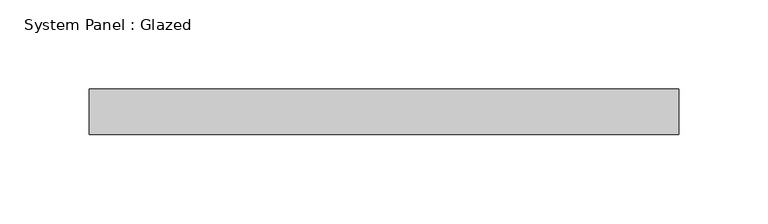
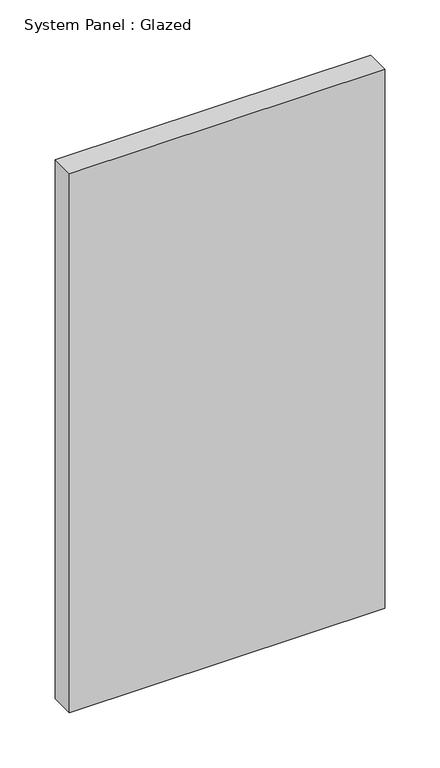
"""IFC4 building model written with IfcOpenShell, lengths in millimetres: plate geometry, System Panel : Glazed."""

from ifc_helpers import new_model, si_unit, origin, origin_with_axes, place, context, project, spatial, polyline, outline, extrude, source, transform, mapped, element, save


def system_panel_glazed_8f64e07d(model_context):
    return source(origin(), model_context, "Body", "SweptSolid", [
        extrude(outline(polyline([(165.1, 19.05), (-165.1, 19.05), (-165.1, 44.45), (165.1, 44.45), (165.1, 19.05)])), origin_with_axes(), (0.0, 0.0, 1.0), 597.0049172),
    ])


if __name__ == "__main__":
    model = new_model("IFC4")
    model_context = context("Model", 3, world=origin())
    ifc_project = project(units=[si_unit("LENGTHUNIT", "METRE", prefix="MILLI")], contexts=[model_context])
    site = spatial("IfcSite", under=ifc_project)
    building = spatial("IfcBuilding", under=site)
    placement = place(None, origin())
    system_panel_glazed_shape = system_panel_glazed_8f64e07d(model_context)
    element("IfcPlate", 1, ObjectType="System Panel : Glazed", at=placement, inside=building, context=model_context, shape_type="MappedRepresentation", body=[
        mapped(system_panel_glazed_shape, transform((0.0, 0.0, 0.0), x_axis=(1.0, 0.0, 0.0), y_axis=(0.0, 1.0, 0.0), z_axis=(0.0, 0.0, 1.0))),
    ])
    save(model, "model.ifc")

# Revit data of these elements
# Type "System Panel : Glazed"
#   Construction Type Id = "GSP4R"
#   Analytic Construction = "1/8 in Pilkington single glazing"
#   Visual Light Transmittance = 0.9
#   Solar Heat Gain Coefficient = 0.86
#   Heat Transfer Coefficient (U) = 1.18115 BTU/(h·ft²·°F)
#   Define Thermal Properties by = 1
# Element 1 (IfcPlate, "System Panel : Glazed")
#   Materials on its faces: "Glass"
# Materials
#   "Glass": class "Glass", colour RGB 0 128 192, transparency 0.75, Description = "Soda Lime Glass", Cost = 0
